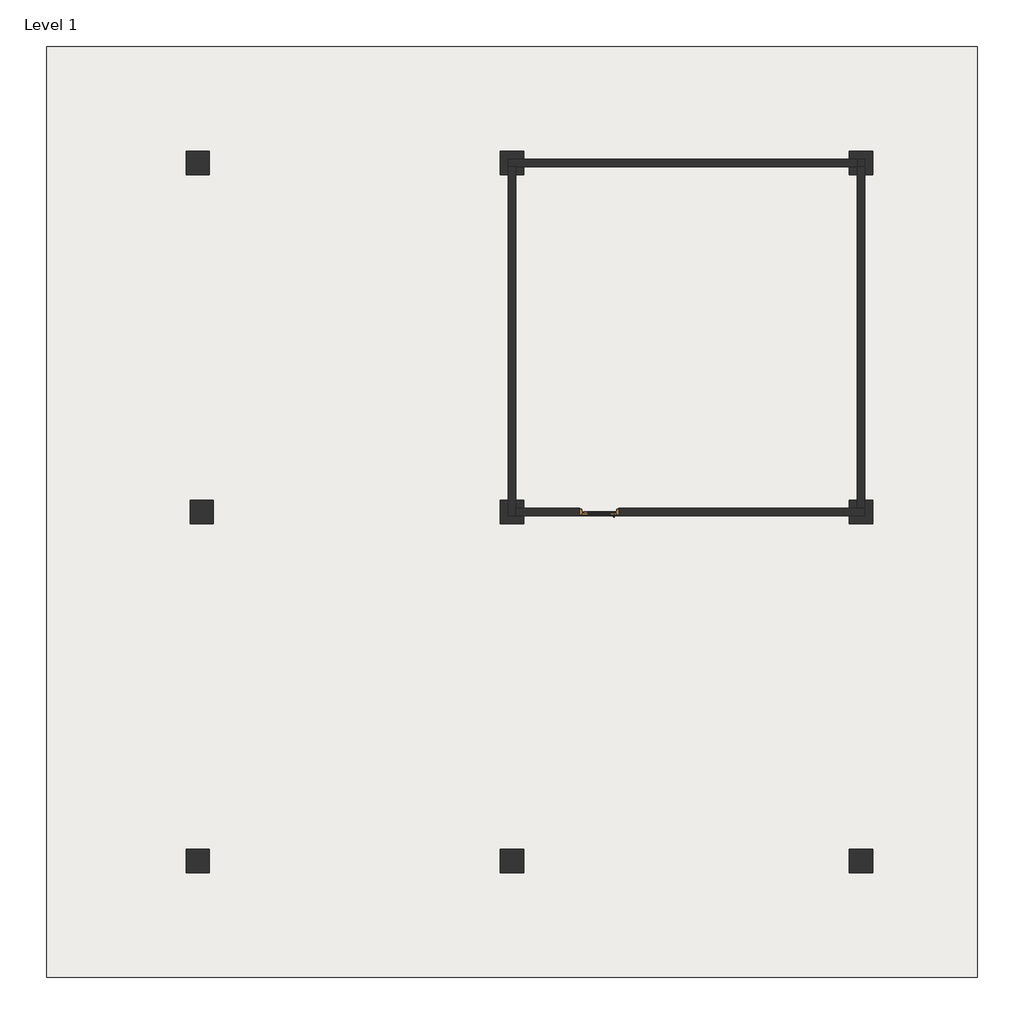
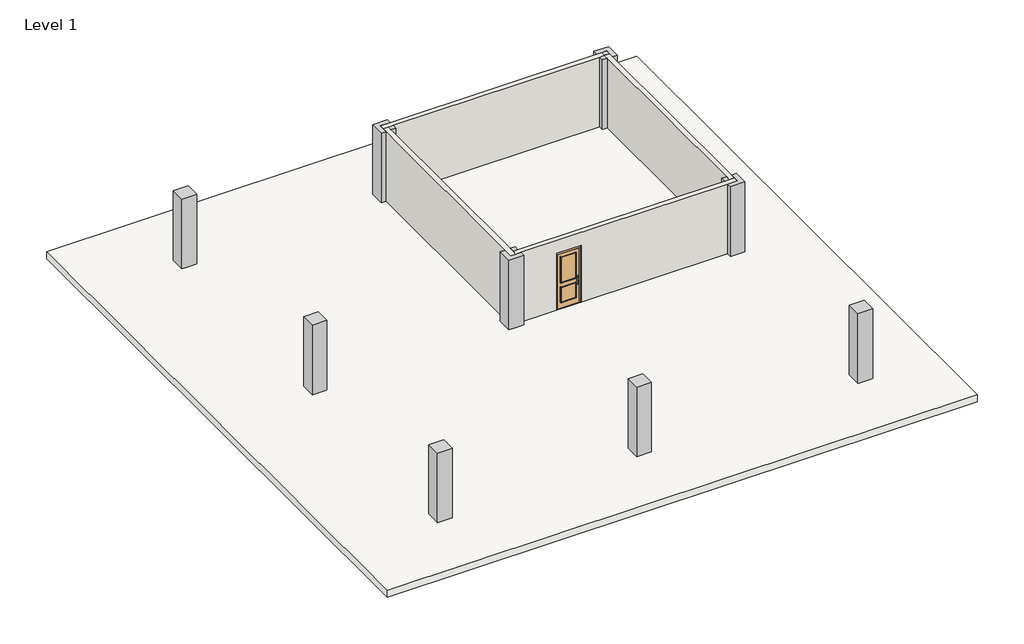
# One storey: 9 columns, 5 walls, 1 door, 1 slab.
"""IFC4 building model written with IfcOpenShell, lengths in millimetres."""

from ifc_helpers import new_model, si_unit, frame, origin, origin_with_axes, place, context, project, spatial, polyline, outline, extrude, faceted_brep, transform, mapped, element, save
from components import door_b6c2ee01

model = new_model("IFC4")

# Units and contexts
model_context = context("Model", 3, world=origin())
ifc_project = project(units=[si_unit("LENGTHUNIT", "METRE", prefix="MILLI")], contexts=[model_context])

# Site, building, storey
site = spatial("IfcSite", under=ifc_project)
building = spatial("IfcBuilding", under=site)
storey = spatial("IfcBuildingStorey", under=building, Name="Level 1", Elevation=0.0)

# Columns
placement = place(None, origin())
element("IfcColumn", 1, ObjectType="Rectangular Column : 24\" x 24\"", at=placement, inside=storey, context=model_context, shape_type="SweptSolid", body=[
    extrude(outline(polyline([(-5575.4937431, 9163.813611), (-5575.4937431, 9773.413611), (-4965.8937431, 9773.413611), (-4965.8937431, 9570.213611), (-5372.2937431, 9570.213611), (-5372.2937431, 9367.013611), (-5372.2937431, 9163.813611), (-5575.4937431, 9163.813611)])), origin_with_axes(), (0.0, 0.0, 1.0), 3048.0),
    extrude(outline(polyline([(-4965.8937431, 9367.013611), (-4965.8937431, 9163.813611), (-5169.0937431, 9163.813611), (-5169.0937431, 9367.013611), (-4965.8937431, 9367.013611)])), origin_with_axes(), (0.0, 0.0, 1.0), 3048.0),
])
element("IfcColumn", 2, ObjectType="Rectangular Column : 24\" x 24\"", at=placement, inside=storey, context=model_context, shape_type="SweptSolid", body=[
    extrude(outline(polyline([(4178.1062569, 9773.413611), (4178.1062569, 9163.813611), (3974.9062569, 9163.813611), (3974.9062569, 9367.013611), (3974.9062569, 9570.213611), (3771.7062569, 9570.213611), (3568.5062569, 9570.213611), (3568.5062569, 9773.413611), (4178.1062569, 9773.413611)])), origin_with_axes(), (0.0, 0.0, 1.0), 3048.0),
    extrude(outline(polyline([(3568.5062569, 9163.813611), (3568.5062569, 9367.013611), (3771.7062569, 9367.013611), (3771.7062569, 9163.813611), (3568.5062569, 9163.813611)])), origin_with_axes(), (0.0, 0.0, 1.0), 3048.0),
])
element("IfcColumn", 3, ObjectType="Rectangular Column : 24\" x 24\"", at=placement, inside=storey, context=model_context, shape_type="SweptSolid", body=[
    extrude(outline(polyline([(-13195.4937431, 9773.413611), (-13195.4937431, 9163.813611), (-13805.0937431, 9163.813611), (-13805.0937431, 9773.413611), (-13195.4937431, 9773.413611)])), origin_with_axes(), (0.0, 0.0, 1.0), 3048.0),
])
element("IfcColumn", 4, ObjectType="Rectangular Column : 24\" x 24\"", at=placement, inside=storey, context=model_context, shape_type="SweptSolid", body=[
    extrude(outline(polyline([(-13093.8937431, 629.413611), (-13093.8937431, 19.813611), (-13703.4937431, 19.813611), (-13703.4937431, 629.413611), (-13093.8937431, 629.413611)])), origin_with_axes(), (0.0, 0.0, 1.0), 3048.0),
])
element("IfcColumn", 5, ObjectType="Rectangular Column : 24\" x 24\"", at=placement, inside=storey, context=model_context, shape_type="SweptSolid", body=[
    extrude(outline(polyline([(3568.5062569, 426.213611), (3568.5062569, 629.413611), (3771.7062569, 629.413611), (3771.7062569, 426.213611), (3568.5062569, 426.213611)])), origin_with_axes(), (0.0, 0.0, 1.0), 3048.0),
    extrude(outline(polyline([(4178.1062569, 629.413611), (4178.1062569, 19.813611), (3568.5062569, 19.813611), (3568.5062569, 223.013611), (3974.9062569, 223.013611), (3974.9062569, 426.213611), (3974.9062569, 629.413611), (4178.1062569, 629.413611)])), origin_with_axes(), (0.0, 0.0, 1.0), 3048.0),
])
element("IfcColumn", 6, ObjectType="Rectangular Column : 24\" x 24\"", at=placement, inside=storey, context=model_context, shape_type="SweptSolid", body=[
    extrude(outline(polyline([(-13195.4937431, -8514.586389), (-13195.4937431, -9124.186389), (-13805.0937431, -9124.186389), (-13805.0937431, -8514.586389), (-13195.4937431, -8514.586389)])), origin_with_axes(), (0.0, 0.0, 1.0), 3048.0),
])
element("IfcColumn", 7, ObjectType="Rectangular Column : 24\" x 24\"", at=placement, inside=storey, context=model_context, shape_type="SweptSolid", body=[
    extrude(outline(polyline([(-4965.8937431, -8514.586389), (-4965.8937431, -9124.186389), (-5575.4937431, -9124.186389), (-5575.4937431, -8514.586389), (-4965.8937431, -8514.586389)])), origin_with_axes(), (0.0, 0.0, 1.0), 3048.0),
])
element("IfcColumn", 8, ObjectType="Rectangular Column : 24\" x 24\"", at=placement, inside=storey, context=model_context, shape_type="SweptSolid", body=[
    extrude(outline(polyline([(4178.1062569, -8514.586389), (4178.1062569, -9124.186389), (3568.5062569, -9124.186389), (3568.5062569, -8514.586389), (4178.1062569, -8514.586389)])), origin_with_axes(), (0.0, 0.0, 1.0), 3048.0),
])
element("IfcColumn", 9, ObjectType="Rectangular Column : 24\" x 24\" 2", at=placement, inside=storey, context=model_context, shape_type="SweptSolid", body=[
    extrude(outline(polyline([(-5169.0937431, 629.413611), (-4965.8937431, 629.413611), (-4965.8937431, 426.213611), (-5169.0937431, 426.213611), (-5169.0937431, 629.413611)])), origin_with_axes(), (0.0, 0.0, 1.0), 3048.0),
    extrude(outline(polyline([(-4965.8937431, 19.813611), (-5575.4937431, 19.813611), (-5575.4937431, 629.413611), (-5372.2937431, 629.413611), (-5372.2937431, 223.013611), (-5169.0937431, 223.013611), (-4965.8937431, 223.013611), (-4965.8937431, 19.813611)])), origin_with_axes(), (0.0, 0.0, 1.0), 3048.0),
])

# Door
door_shape = door_b6c2ee01(model_context)
element("IfcDoor", 10, ObjectType="Door-Exterior-Single-Two_Lite : 36\" x 94\"", at=placement, inside=storey, context=model_context, shape_type="MappedRepresentation", body=[
    mapped(door_shape, transform((-2984.6937431, 330.963611, 0.0), x_axis=(-1.0, 0.0, 0.0), y_axis=(0.0, -1.0, 0.0), z_axis=(0.0, 0.0, 1.0))),
])

# Slab
element("IfcSlab", 11, ObjectType="Generic - 12\" - Filled 2", at=placement, inside=storey, context=model_context, shape_type="SweptSolid", body=[
    extrude(outline(polyline([(6921.3062569, 12516.613611), (6921.3062569, -11867.386389), (-17462.6937431, -11867.386389), (-17462.6937431, 12516.613611), (6921.3062569, 12516.613611)])), frame((0.0, 0.0, -304.8), z_axis=(0.0, 0.0, 1.0), x_axis=(1.0, 0.0, 0.0)), (0.0, 0.0, 1.0), 304.8),
])

# Walls
element("IfcWall", 12, ObjectType="Generic - 8\" 2", at=placement, inside=storey, context=model_context, shape_type="Brep", body=[
    faceted_brep([(-5372.2937431, 9367.013611, 0.0), (-5169.0937431, 9367.013611, 0.0), (-4965.8937431, 9367.013611, 0.0), (3568.5062569, 9367.013611, 0.0), (3771.7062569, 9367.013611, 0.0), (3771.7062569, 9367.013611, 3048.0), (3568.5062569, 9367.013611, 3048.0), (-4965.8937431, 9367.013611, 3048.0), (-5169.0937431, 9367.013611, 3048.0), (-5372.2937431, 9367.013611, 3048.0), (-5372.2937431, 9570.213611, 0.0), (-5372.2937431, 9570.213611, 3048.0), (-4965.8937431, 9570.213611, 3048.0), (3568.5062569, 9570.213611, 3048.0), (3771.7062569, 9570.213611, 3048.0), (3771.7062569, 9570.213611, 0.0), (3568.5062569, 9570.213611, 0.0), (-4965.8937431, 9570.213611, 0.0)], [[[0, 1, 2, 3, 4, 5, 6, 7, 8, 9]], [[10, 11, 12, 13, 14, 15, 16, 17]], [[4, 3, 2, 1, 0, 10, 17, 16, 15]], [[9, 8, 7, 6, 5, 14, 13, 12, 11]], [[0, 9, 11, 10]], [[5, 4, 15, 14]]]),
])
element("IfcWall", 13, ObjectType="Generic - 8\" 2", at=placement, inside=storey, context=model_context, shape_type="Brep", body=[
    faceted_brep([(-5169.0937431, 223.013611, 0.0), (-5169.0937431, 426.213611, 0.0), (-5169.0937431, 629.413611, 0.0), (-5169.0937431, 9163.813611, 0.0), (-5169.0937431, 9367.013611, 0.0), (-5169.0937431, 9367.013611, 3048.0), (-5169.0937431, 9163.813611, 3048.0), (-5169.0937431, 629.413611, 3048.0), (-5169.0937431, 426.213611, 3048.0), (-5169.0937431, 223.013611, 3048.0), (-5372.2937431, 223.013611, 0.0), (-5372.2937431, 223.013611, 3048.0), (-5372.2937431, 629.413611, 3048.0), (-5372.2937431, 9163.813611, 3048.0), (-5372.2937431, 9367.013611, 3048.0), (-5372.2937431, 9367.013611, 0.0), (-5372.2937431, 9163.813611, 0.0), (-5372.2937431, 629.413611, 0.0)], [[[0, 1, 2, 3, 4, 5, 6, 7, 8, 9]], [[10, 11, 12, 13, 14, 15, 16, 17]], [[4, 3, 2, 1, 0, 10, 17, 16, 15]], [[9, 8, 7, 6, 5, 14, 13, 12, 11]], [[0, 9, 11, 10]], [[5, 4, 15, 14]]]),
])
element("IfcWall", 14, ObjectType="Generic - 8\" 4", at=placement, inside=storey, context=model_context, shape_type="Brep", body=[
    faceted_brep([(-5169.0937431, 426.213611, 3048.0), (-4965.8937431, 426.213611, 3048.0), (3568.5062569, 426.213611, 3048.0), (3771.7062569, 426.213611, 3048.0), (3974.9062569, 426.213611, 3048.0), (3974.9062569, 426.213611, 0.0), (3771.7062569, 426.213611, 0.0), (3568.5062569, 426.213611, 0.0), (-2476.6937431, 426.213611, 0.0), (-2476.6937431, 426.213611, 2489.2), (-3492.6937431, 426.213611, 2489.2), (-3492.6937431, 426.213611, 0.0), (-4965.8937431, 426.213611, 0.0), (-5169.0937431, 426.213611, 0.0), (3974.9062569, 223.013611, 3048.0), (3568.5062569, 223.013611, 3048.0), (-4965.8937431, 223.013611, 3048.0), (-5169.0937431, 223.013611, 3048.0), (-5169.0937431, 223.013611, 0.0), (-4965.8937431, 223.013611, 0.0), (-3492.6937431, 223.013611, 0.0), (-3492.6937431, 223.013611, 2489.2), (-2476.6937431, 223.013611, 2489.2), (-2476.6937431, 223.013611, 0.0), (3568.5062569, 223.013611, 0.0), (3974.9062569, 223.013611, 0.0)], [[[0, 1, 2, 3, 4, 5, 6, 7, 8, 9, 10, 11, 12, 13]], [[14, 15, 16, 17, 18, 19, 20, 21, 22, 23, 24, 25]], [[18, 13, 12, 11, 20, 19]], [[5, 25, 24, 23, 8, 7, 6]], [[4, 3, 2, 1, 0, 17, 16, 15, 14]], [[5, 4, 14, 25]], [[0, 13, 18, 17]], [[10, 21, 20, 11]], [[21, 10, 9, 22]], [[22, 9, 8, 23]]]),
])
element("IfcWall", 15, ObjectType="Generic - 8\" 4", at=placement, inside=storey, context=model_context, shape_type="SweptSolid", body=[
    extrude(outline(polyline([(3771.7062569, 9367.013611), (3771.7062569, 9570.213611), (3974.9062569, 9570.213611), (3974.9062569, 9367.013611), (3771.7062569, 9367.013611)])), origin_with_axes(), (0.0, 0.0, 1.0), 3048.0),
])
element("IfcWall", 16, ObjectType="Generic - 8\" 4", at=placement, inside=storey, context=model_context, shape_type="Brep", body=[
    faceted_brep([(3771.7062569, 9367.013611, 0.0), (3771.7062569, 9163.813611, 0.0), (3771.7062569, 629.413611, 0.0), (3771.7062569, 426.213611, 0.0), (3771.7062569, 426.213611, 3048.0), (3771.7062569, 629.413611, 3048.0), (3771.7062569, 9163.813611, 3048.0), (3771.7062569, 9367.013611, 3048.0), (3974.9062569, 9367.013611, 0.0), (3974.9062569, 9367.013611, 3048.0), (3974.9062569, 9163.813611, 3048.0), (3974.9062569, 629.413611, 3048.0), (3974.9062569, 426.213611, 3048.0), (3974.9062569, 426.213611, 0.0), (3974.9062569, 629.413611, 0.0), (3974.9062569, 9163.813611, 0.0)], [[[0, 1, 2, 3, 4, 5, 6, 7]], [[8, 9, 10, 11, 12, 13, 14, 15]], [[3, 2, 1, 0, 8, 15, 14, 13]], [[7, 6, 5, 4, 12, 11, 10, 9]], [[0, 7, 9, 8]], [[4, 3, 13, 12]]]),
])

save(model, "model.ifc")

# Revit data of these elements
# Type "Rectangular Column : 24\" x 24\""
#   Assembly Code = "B1010200"
#   Depth = 2' - 0"
#   Offset Base = 0' - 0"
#   Offset Top = 0' - 0"
#   Width = 2' - 0"
#   built-in parameter 1002110 = 16777215
#   Material = Parking Stripe
# Type "Rectangular Column : 24\" x 24\" 2"
#   Assembly Code = "B1010200"
#   Depth = 2' - 0"
#   Offset Base = 0' - 0"
#   Offset Top = 0' - 0"
#   Width = 2' - 0"
#   built-in parameter 1002110 = 16777215
#   Material = Parking Stripe
# Type "Door-Exterior-Single-Two_Lite : 36\" x 94\""
#   Type Mark = "9"
#   Assembly Code = "B2030100"
#   Analytic Construction = "Metal frame, double glass door"
#   Top Rail = 0' - 6"
#   Threshold Offset [instance default] = 0' - 0 1/2"
#   Threshold Length [instance default] = 3' - 4"
#   Thickness = 0' - 1 3/4"
#   Thermal Resistance (R) = 1.3794 (h·ft²·°F)/BTU
#   Swing Angle [instance default] = 90.00°
#   Strike Height = 3' - 4"
#   Stiles = 0' - 6"
#   Rough Width [instance default] = 3' - 4"
#   Rough Height [instance default] = 8' - 2"
#   MFOpeningHeight [instance default] = 0' - 4"
#   MFOpeningWidth [instance default] = 0' - 4"
#   Lock Rail = 0' - 7 1/2"
#   Heat Transfer Coefficient (U) = 0.7250 BTU/(h·ft²·°F)
#   Glass Thickness = 0' - 0 3/4"
#   Inset Calculate [instance default] = 0' - 4"
#   Masonry Inset [instance default] = 0' - 1"
#   Height = 7' - 10"
#   Width = 3' - 0"
#   Masonry Frame Depth = 0' - 5 3/4"
#   Bottom Rail = 0' - 10"
#   Masonry Frame [instance default] = yes
#   Function = 1
#   Threshold [instance default] = yes
#   Dry Wall Frame [instance default] = no
#   Threshold Material = none
#   Panic Bar Material = Metal - Stainless Steel
#   Panel Material = Metal - Painted - Grey
#   Glass Stop Material = Metal - Painted - Grey
#   Exterior Pull Material = Metal - Stainless Steel
#   Frame Material = Metal - Painted - Grey
#   Visual Light Transmittance = 0
#   Solar Heat Gain Coefficient = 0
#   Wall Closure = (empty or 0)
# Type "Generic - 12\" - Filled 2"
#   Assembly Code = "B1010"
#   Function = 0
#   Layers, outside or top first: 1' - 0" "Parking Stripe" (function 1)
# Type "Generic - 8\" 2"
#   Assembly Code = "B2010"
#   Layers, outside or top first: 0' - 8" "Parking Stripe" (function 1)
# Type "Generic - 8\" 4"
#   Assembly Code = "B2010"
#   Layers, outside or top first: 0' - 8" "Parking Stripe" (function 1)
# Elements 1, 2, 5 (IfcColumn, "Rectangular Column : 24\" x 24\"")
#   Phase Created = New Construction
#   Materials on its faces: "Parking Stripe", "Gypsum Wall Board"
# Elements 3, 4, 6, 7, 8 (IfcColumn, "Rectangular Column : 24\" x 24\"")
#   Phase Created = New Construction
#   Materials on its faces: "Gypsum Wall Board", "Parking Stripe"
# Element 9 (IfcColumn, "Rectangular Column : 24\" x 24\" 2")
#   Phase Created = New Construction
#   Materials on its faces: "Parking Stripe", "Gypsum Wall Board"
# Element 10 (IfcDoor, "Door-Exterior-Single-Two_Lite : 36\" x 94\"")
#   Threshold Offset = 0' - 0 1/2"
#   Threshold Length = 3' - 4"
#   Swing Angle = 90.00°
#   Rough Width = 3' - 4"
#   Rough Height = 8' - 2"
#   Masonry Inset = 0' - 1"
#   MFOpeningWidth = 0' - 4"
#   MFOpeningHeight = 0' - 4"
#   Inset Calculate = 0' - 4"
#   Threshold = yes
#   Masonry Frame = yes
#   Dry Wall Frame = no
#   Phase Created = New Construction
#   Materials on its faces: "Metal - Painted - Grey", "Metal - Stainless Steel", "Glass"
# Element 11 (IfcSlab, "Generic - 12\" - Filled 2")
#   Height Offset From Level = 0' - 0"
#   Phase Created = New Construction
#   Materials on its faces: "Gypsum Wall Board", "Parking Stripe"
# Elements 12, 13 (IfcWall, "Generic - 8\" 2")
#   Top Offset = 0' - 0"
#   Base Offset = 0' - 0"
#   Unconnected Height = 10' - 0"
#   wall height = 10' - 0"
#   Phase Created = New Construction
#   Base Constraint = Level 1
#   Materials on its faces: "Parking Stripe"
# Elements 14, 15, 16 (IfcWall, "Generic - 8\" 4")
#   Top Offset = 0' - 0"
#   Base Offset = 0' - 0"
#   Unconnected Height = 10' - 0"
#   wall height = 10' - 0"
#   Phase Created = New Construction
#   Base Constraint = Level 1
#   Materials on its faces: "Parking Stripe"
# Materials
#   "Parking Stripe": class "Paint", colour RGB 250 250 91, transparency 0, Cost = 0
#   "Metal - Stainless Steel": class "Metal", colour RGB 247 247 247, transparency 0
#   "Metal - Painted - Grey": class "Paint", colour RGB 104 104 104, transparency 0
#   "Gypsum Wall Board": class "Generic", colour RGB 127 127 127, transparency 0, Description = "Gypsum Wall Board", Cost = 0
#   "Glass": class "Glass", colour RGB 0 128 192, transparency 0.75, Description = "Soda Lime Glass", Cost = 0
